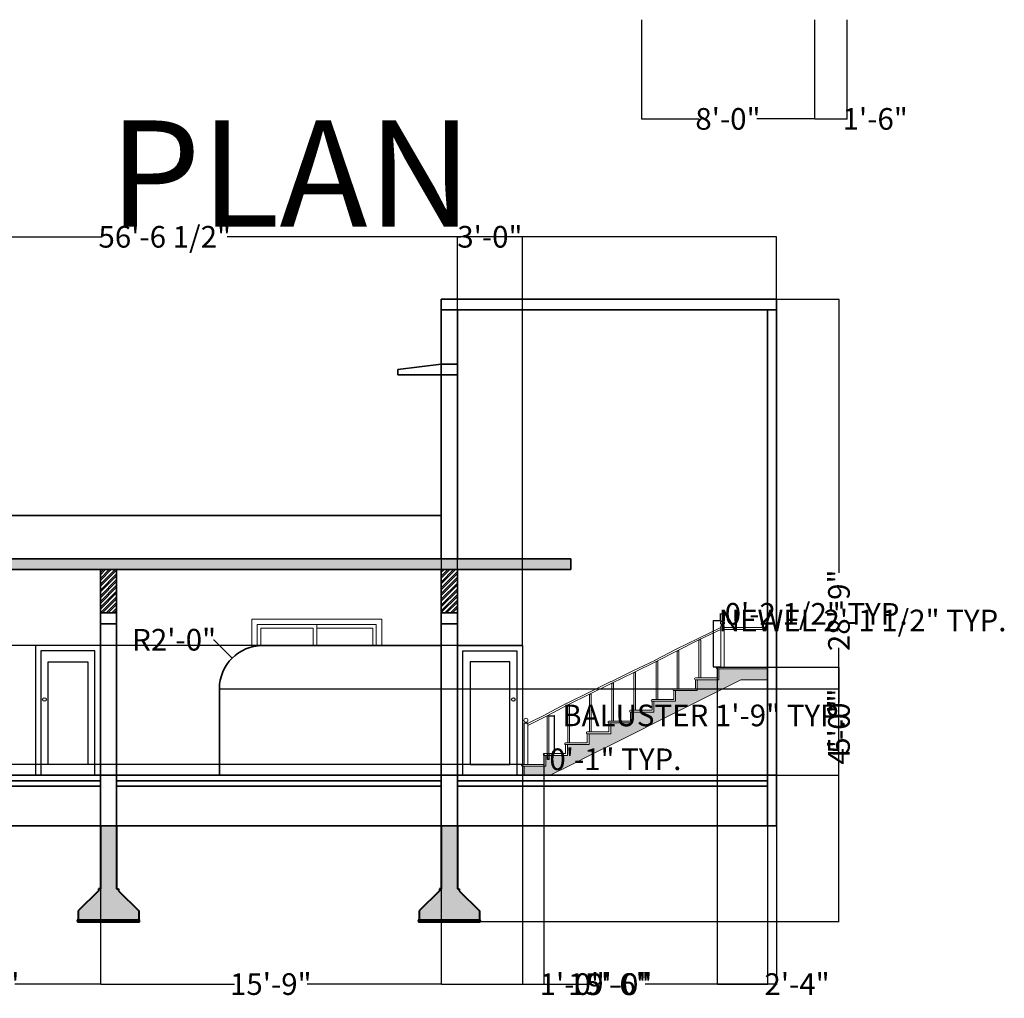
# Model space of a CAD drawing. Units: inches. Extents: x 1146 to 2917, y 889 to 2437.
# Tile 2 of 13: x 1551 to 2097, y 889 to 1432. Entities that reach past the tile are written whole.
import ezdxf

# ---------------------------------------------------------------- set-up
doc = ezdxf.new("R2010")
doc.units = ezdxf.units.IN
doc.header["$MEASUREMENT"] = 0
for name, color, linetype, lineweight in [('A-ANNO-DIMS', 2, 'Continuous', 18), ('A-ANNO-TEXT', 7, 'Continuous', 25), ('A-SECT', 7, 'Continuous', 35), ('A-SECT-PATT', 8, 'Continuous', 13), ('A-SECT-STRS', 6, 'Continuous', 20), ('door', 10, 'Continuous', 25), ('S-FNDN', 7, 'Continuous', 40), ('window', 5, 'Continuous', 18)]:
    doc.layers.add(name, color=color, linetype=linetype, lineweight=lineweight)
doc.styles.get("Standard").update_dxf_attribs({"font": 'arial.ttf'})
doc.dimstyles.get("Standard").update_dxf_attribs({"dimtxt": 12, "dimasz": 0.18, "dimexe": 0.18, "dimexo": 0.0625, "dimgap": 0.09, "dimtad": 0, "dimtoh": 1, "dimdec": 1, "dimzin": 0, "dimdsep": 46, "dimlunit": 4, "dimtxsty": 'Standard', "dimcen": 0.09, "dimadec": 0, "dimazin": 0, "dimtfac": 1, "dimtdec": 1, "dimtofl": 0, "dimtmove": 0, "dimatfit": 3, "dimfxl": 1, "dimtolj": 1, "dimtzin": 0, "dimarcsym": 0})

# ---------------------------------------------------------------- blocks, each defined once
blk = doc.blocks.new('*U61')
blk.add_lwpolyline([(3.12, 0.01), (0.12, 0.01), (0.12, 72.01), (36.12, 72.01), (36.12, 0.01), (33.12, 0.01)])
for points in [[(33.12, 68.99), (33.12, 0.01), (3.12, 0.01), (3.12, 68.99)], [(29.12, 6.01), (29.12, 62.99), (7.12, 62.99), (7.12, 6.01)]]:
    blk.add_lwpolyline(points, close=True)
blk.add_circle((31.12, 42.01), 1)
blk = doc.blocks.new('*U62')
blk.add_lwpolyline([(-6.87, 0.01), (-3.87, 0.01), (-3.87, 72.01), (-39.87, 72.01), (-39.87, 0.01), (-36.87, 0.01)])
for points in [[(-36.87, 68.99), (-36.87, 0.01), (-6.87, 0.01), (-6.87, 68.99)], [(-32.87, 6.01), (-32.87, 62.99), (-10.87, 62.99), (-10.87, 6.01)]]:
    blk.add_lwpolyline(points, close=True)
blk.add_circle((-34.87, 42.01), 1)
blk = doc.blocks.new('RAILING-BALUSTER')
for p, q in [((0, 0), (0, 21)), ((0, 21), (1, 21)), ((1, 21), (1, 0))]:
    blk.add_line(p, q)
blk = doc.blocks.new('RAILING-NEWEL')
for p, q in [((0.13, 23.99), (0.13, 24)), ((0.13, 12), (0.13, 22.87)), ((0.13, 22.87), (2.13, 22.87)), ((0.63, 22.87), (0.63, 23.5)), ((1.63, 22.87), (1.63, 23.5)), ((2.13, 24), (2.13, 23.99)), ((2.13, 22.87), (2.13, 0)), ((0.13, 0), (0.13, 12))]:
    blk.add_line(p, q)
blk.add_circle((1.13, 24.51), 1.13)
blk = doc.blocks.new('*D93')
at = {"layer": 'A-ANNO-DIMS', "color": 0, "lineweight": -2, "transparency": 16777216}
for p, q in [((1844.94, 1045.97), (1848.21, 1045.97)), ((1848.03, 1045.97), (1848.03, 1046.15)), ((1848.03, 1046.15), (1848.21, 1046.15)), ((1848.03, 1025.15), (1848.03, 1045.79)), ((1844.94, 1024.97), (1848.21, 1024.97))]:
    blk.add_line(p, q, dxfattribs=at)
at = {"layer": 'A-ANNO-DIMS', "color": 0, "transparency": 16777216}
for points in [[(1848, 1045.79), (1848.06, 1045.79), (1848.03, 1045.97)], [(1848, 1025.15), (1848.06, 1025.15), (1848.03, 1024.97)]]:
    blk.add_solid(points, dxfattribs=at)
at = {"layer": 'Defpoints', "color": 0, "transparency": 16777216}
for p in [(1844.88, 1045.97), (1848.03, 1045.97), (1844.88, 1024.97)]:
    blk.add_point(p, dxfattribs=at)
at = {"layer": 'A-ANNO-DIMS', "color": 0, "transparency": 16777216, "insert": (1931.19, 1046.15), "char_height": 12, "attachment_point": 5}
blk.add_mtext('\\A1;BALUSTER 1\'-9" TYP.', dxfattribs=at)
blk = doc.blocks.new('*D94')
at = {"layer": 'A-ANNO-DIMS', "color": 0, "lineweight": -2, "transparency": 16777216}
for p, q in [((1843.88, 1024.9), (1843.88, 1021.64)), ((1844.06, 1021.82), (1844.7, 1021.82)), ((1844.88, 1024.9), (1844.88, 1021.64)), ((1844.88, 1021.82), (1845.06, 1021.82))]:
    blk.add_line(p, q, dxfattribs=at)
at = {"layer": 'A-ANNO-DIMS', "color": 0, "transparency": 16777216}
for points in [[(1844.06, 1021.85), (1844.06, 1021.79), (1843.88, 1021.82)], [(1844.7, 1021.85), (1844.7, 1021.79), (1844.88, 1021.82)]]:
    blk.add_solid(points, dxfattribs=at)
at = {"layer": 'Defpoints', "color": 0, "transparency": 16777216}
for p in [(1843.88, 1024.97), (1844.88, 1024.97), (1844.88, 1021.82)]:
    blk.add_point(p, dxfattribs=at)
at = {"layer": 'A-ANNO-DIMS', "color": 0, "transparency": 16777216, "insert": (1881.72, 1021.82), "char_height": 12, "attachment_point": 5}
blk.add_mtext('\\A1;0\'-1" TYP.', dxfattribs=at)
blk = doc.blocks.new('*D95')
at = {"layer": 'A-ANNO-DIMS', "color": 0, "lineweight": -2, "transparency": 16777216}
for p, q in [((1939.92, 1098.61), (1935.95, 1098.61)), ((1936.13, 1098.61), (1936.13, 1098.79)), ((1936.13, 1098.79), (1936.31, 1098.79)), ((1936.13, 1073.15), (1936.13, 1098.43)), ((1939.92, 1072.97), (1935.95, 1072.97))]:
    blk.add_line(p, q, dxfattribs=at)
at = {"layer": 'A-ANNO-DIMS', "color": 0, "transparency": 16777216}
for points in [[(1936.1, 1098.43), (1936.16, 1098.43), (1936.13, 1098.61)], [(1936.1, 1073.15), (1936.16, 1073.15), (1936.13, 1072.97)]]:
    blk.add_solid(points, dxfattribs=at)
at = {"layer": 'Defpoints', "color": 0, "transparency": 16777216}
for p in [(1936.13, 1098.61), (1939.98, 1098.61), (1939.98, 1072.97)]:
    blk.add_point(p, dxfattribs=at)
at = {"layer": 'A-ANNO-DIMS', "color": 0, "transparency": 16777216, "insert": (2018.8, 1098.79), "char_height": 12, "attachment_point": 5}
blk.add_mtext('\\A1;NEWEL 2\'-1 1/2" TYP.', dxfattribs=at)
blk = doc.blocks.new('*D96')
at = {"layer": 'A-ANNO-DIMS', "color": 0, "lineweight": -2, "transparency": 16777216}
for p, q in [((1939.98, 1098.67), (1939.98, 1102.64)), ((1940.16, 1102.46), (1942.06, 1102.46)), ((1942.24, 1098.67), (1942.24, 1102.64)), ((1942.24, 1102.46), (1942.42, 1102.46))]:
    blk.add_line(p, q, dxfattribs=at)
at = {"layer": 'A-ANNO-DIMS', "color": 0, "transparency": 16777216}
for points in [[(1940.16, 1102.49), (1940.16, 1102.43), (1939.98, 1102.46)], [(1942.06, 1102.49), (1942.06, 1102.43), (1942.24, 1102.46)]]:
    blk.add_solid(points, dxfattribs=at)
at = {"layer": 'Defpoints', "color": 0, "transparency": 16777216}
for p in [(1939.98, 1098.61), (1942.24, 1102.46), (1942.24, 1098.61)]:
    blk.add_point(p, dxfattribs=at)
at = {"layer": 'A-ANNO-DIMS', "color": 0, "transparency": 16777216, "insert": (1993.06, 1102.46), "char_height": 12, "attachment_point": 5}
blk.add_mtext('\\A1;0\'-2 1/2" TYP.', dxfattribs=at)
blk = doc.blocks.new('*D141')
at = {"layer": 'A-ANNO-DIMS', "color": 0, "lineweight": -2, "transparency": 16777216}
for p, q in [((1292.5, 931.94), (1292.5, 1311.7)), ((1292.68, 1311.52), (1597.13, 1311.52)), ((1970.95, 1311.52), (1666.5, 1311.52)), ((1971.13, 1277.03), (1971.13, 1311.7))]:
    blk.add_line(p, q, dxfattribs=at)
at = {"layer": 'A-ANNO-DIMS', "color": 0, "transparency": 16777216}
for points in [[(1292.68, 1311.55), (1292.68, 1311.49), (1292.5, 1311.52)], [(1970.95, 1311.55), (1970.95, 1311.49), (1971.13, 1311.52)]]:
    blk.add_solid(points, dxfattribs=at)
at = {"layer": 'Defpoints', "color": 0, "transparency": 16777216}
for p in [(1971.13, 1311.52), (1971.13, 1276.97), (1292.5, 931.87)]:
    blk.add_point(p, dxfattribs=at)
at = {"layer": 'A-ANNO-DIMS', "color": 0, "transparency": 16777216, "insert": (1631.82, 1311.52), "char_height": 12, "attachment_point": 5}
blk.add_mtext('\\A1;56\'-6 1/2"', dxfattribs=at)
blk = doc.blocks.new('*D142')
at = {"layer": 'A-ANNO-DIMS', "color": 0, "lineweight": -2, "transparency": 16777216}
for p, q in [((1785.2, 1276.97), (2005.86, 1276.97)), ((2005.68, 1276.79), (2005.68, 1125.22)), ((2005.68, 932.05), (2005.68, 1083.62)), ((1806.83, 931.87), (2005.86, 931.87))]:
    blk.add_line(p, q, dxfattribs=at)
at = {"layer": 'A-ANNO-DIMS', "color": 0, "transparency": 16777216}
for points in [[(2005.65, 1276.79), (2005.71, 1276.79), (2005.68, 1276.97)], [(2005.65, 932.05), (2005.71, 932.05), (2005.68, 931.87)]]:
    blk.add_solid(points, dxfattribs=at)
at = {"layer": 'Defpoints', "color": 0, "transparency": 16777216}
for p in [(1785.13, 1276.97), (1806.77, 931.87), (2005.68, 931.87)]:
    blk.add_point(p, dxfattribs=at)
at = {"layer": 'A-ANNO-DIMS', "color": 0, "transparency": 16777216, "insert": (2005.68, 1104.42), "char_height": 12, "attachment_point": 5, "rotation": 90}
blk.add_mtext('\\A1;28\'-9"', dxfattribs=at)
blk = doc.blocks.new('*D147')
at = {"layer": 'A-ANNO-DIMS', "color": 0, "lineweight": -2, "transparency": 16777216}
for p, q in [((1461.13, 984.9), (1461.13, 897)), ((1596.13, 984.9), (1596.13, 897)), ((1461.31, 897.18), (1508.5, 897.18)), ((1595.95, 897.18), (1548.77, 897.18))]:
    blk.add_line(p, q, dxfattribs=at)
at = {"layer": 'A-ANNO-DIMS', "color": 0, "transparency": 16777216}
for points in [[(1461.31, 897.21), (1461.31, 897.15), (1461.13, 897.18)], [(1595.95, 897.21), (1595.95, 897.15), (1596.13, 897.18)]]:
    blk.add_solid(points, dxfattribs=at)
at = {"layer": 'Defpoints', "color": 0, "transparency": 16777216}
for p in [(1461.13, 984.97), (1596.13, 984.97), (1596.13, 897.18)]:
    blk.add_point(p, dxfattribs=at)
at = {"layer": 'A-ANNO-DIMS', "color": 0, "transparency": 16777216, "insert": (1528.63, 897.18), "char_height": 12, "attachment_point": 5}
blk.add_mtext('\\A1;11\'-3"', dxfattribs=at)
blk = doc.blocks.new('*D148')
at = {"layer": 'A-ANNO-DIMS', "color": 0, "lineweight": -2, "transparency": 16777216}
for p, q in [((1596.13, 984.9), (1596.13, 897)), ((1785.13, 984.9), (1785.13, 897)), ((1596.31, 897.18), (1670.5, 897.18)), ((1784.95, 897.18), (1710.77, 897.18))]:
    blk.add_line(p, q, dxfattribs=at)
at = {"layer": 'A-ANNO-DIMS', "color": 0, "transparency": 16777216}
for points in [[(1596.31, 897.21), (1596.31, 897.15), (1596.13, 897.18)], [(1784.95, 897.21), (1784.95, 897.15), (1785.13, 897.18)]]:
    blk.add_solid(points, dxfattribs=at)
at = {"layer": 'Defpoints', "color": 0, "transparency": 16777216}
for p in [(1596.13, 984.97), (1785.13, 984.97), (1785.13, 897.18)]:
    blk.add_point(p, dxfattribs=at)
at = {"layer": 'A-ANNO-DIMS', "color": 0, "transparency": 16777216, "insert": (1690.63, 897.18), "char_height": 12, "attachment_point": 5}
blk.add_mtext('\\A1;15\'-9"', dxfattribs=at)
blk = doc.blocks.new('*D149')
at = {"layer": 'A-ANNO-DIMS', "color": 0, "lineweight": -2, "transparency": 16777216}
for p, q in [((1785.13, 1276.9), (1785.13, 897)), ((1971.13, 1276.9), (1971.13, 897)), ((1785.31, 897.18), (1858, 897.18)), ((1970.95, 897.18), (1898.27, 897.18))]:
    blk.add_line(p, q, dxfattribs=at)
at = {"layer": 'A-ANNO-DIMS', "color": 0, "transparency": 16777216}
for points in [[(1785.31, 897.21), (1785.31, 897.15), (1785.13, 897.18)], [(1970.95, 897.21), (1970.95, 897.15), (1971.13, 897.18)]]:
    blk.add_solid(points, dxfattribs=at)
at = {"layer": 'Defpoints', "color": 0, "transparency": 16777216}
for p in [(1785.13, 1276.97), (1971.13, 1276.97), (1971.13, 897.18)]:
    blk.add_point(p, dxfattribs=at)
at = {"layer": 'A-ANNO-DIMS', "color": 0, "transparency": 16777216, "insert": (1878.13, 897.18), "char_height": 12, "attachment_point": 5}
blk.add_mtext('\\A1;15\'-6"', dxfattribs=at)
blk = doc.blocks.new('*D151')
at = {"layer": 'A-ANNO-DIMS', "color": 0, "lineweight": -2, "transparency": 16777216}
for p, q in [((1938.2, 1072.97), (2005.86, 1072.97)), ((2005.68, 1072.79), (2005.68, 1059.01)), ((2005.68, 1013.15), (2005.68, 1026.93)), ((1830.2, 1012.97), (2005.86, 1012.97))]:
    blk.add_line(p, q, dxfattribs=at)
at = {"layer": 'A-ANNO-DIMS', "color": 0, "transparency": 16777216}
for points in [[(2005.65, 1072.79), (2005.71, 1072.79), (2005.68, 1072.97)], [(2005.65, 1013.15), (2005.71, 1013.15), (2005.68, 1012.97)]]:
    blk.add_solid(points, dxfattribs=at)
at = {"layer": 'Defpoints', "color": 0, "transparency": 16777216}
for p in [(1938.13, 1072.97), (2005.68, 1072.97), (1830.13, 1012.97)]:
    blk.add_point(p, dxfattribs=at)
at = {"layer": 'A-ANNO-DIMS', "color": 0, "transparency": 16777216, "insert": (2005.68, 1042.97), "char_height": 12, "attachment_point": 5, "rotation": 90}
blk.add_mtext('\\A1;5\'-0"', dxfattribs=at)
blk = doc.blocks.new('*D152')
at = {"layer": 'A-ANNO-DIMS', "color": 0, "lineweight": -2, "transparency": 16777216}
for p, q in [((1938.13, 1072.9), (1938.13, 897)), ((1830.13, 1012.9), (1830.13, 897)), ((1830.31, 897.18), (1868.09, 897.18)), ((1937.95, 897.18), (1900.17, 897.18))]:
    blk.add_line(p, q, dxfattribs=at)
at = {"layer": 'A-ANNO-DIMS', "color": 0, "transparency": 16777216}
for points in [[(1830.31, 897.21), (1830.31, 897.15), (1830.13, 897.18)], [(1937.95, 897.21), (1937.95, 897.15), (1938.13, 897.18)]]:
    blk.add_solid(points, dxfattribs=at)
at = {"layer": 'Defpoints', "color": 0, "transparency": 16777216}
for p in [(1938.13, 1072.97), (1830.13, 1012.97), (1938.13, 897.18)]:
    blk.add_point(p, dxfattribs=at)
at = {"layer": 'A-ANNO-DIMS', "color": 0, "transparency": 16777216, "insert": (1884.13, 897.18), "char_height": 12, "attachment_point": 5}
blk.add_mtext('\\A1;9\'-0"', dxfattribs=at)
blk = doc.blocks.new('*D153')
at = {"layer": 'A-ANNO-DIMS', "color": 0, "lineweight": -2, "transparency": 16777216}
for p, q in [((1938.13, 1072.9), (1938.13, 897)), ((1966.13, 1072.9), (1966.13, 897)), ((1938.31, 897.18), (1965.95, 897.18)), ((1966.13, 897.18), (1966.31, 897.18))]:
    blk.add_line(p, q, dxfattribs=at)
at = {"layer": 'A-ANNO-DIMS', "color": 0, "transparency": 16777216}
for points in [[(1938.31, 897.21), (1938.31, 897.15), (1938.13, 897.18)], [(1965.95, 897.21), (1965.95, 897.15), (1966.13, 897.18)]]:
    blk.add_solid(points, dxfattribs=at)
at = {"layer": 'Defpoints', "color": 0, "transparency": 16777216}
for p in [(1938.13, 1072.97), (1966.13, 1072.97), (1966.13, 897.18)]:
    blk.add_point(p, dxfattribs=at)
at = {"layer": 'A-ANNO-DIMS', "color": 0, "transparency": 16777216, "insert": (1982.46, 897.18), "char_height": 12, "attachment_point": 5}
blk.add_mtext('\\A1;2\'-4"', dxfattribs=at)
blk = doc.blocks.new('*D154')
at = {"layer": 'A-ANNO-DIMS', "color": 0, "lineweight": -2, "transparency": 16777216}
for p, q in [((1830.07, 1018.97), (1257.62, 1018.97)), ((1257.8, 1018.97), (1257.8, 1019.15)), ((1257.8, 1019.15), (1257.98, 1019.15)), ((1257.8, 1013.15), (1257.8, 1018.79)), ((1830.07, 1012.97), (1257.62, 1012.97))]:
    blk.add_line(p, q, dxfattribs=at)
at = {"layer": 'A-ANNO-DIMS', "color": 0, "transparency": 16777216}
for points in [[(1257.77, 1018.79), (1257.83, 1018.79), (1257.8, 1018.97)], [(1257.77, 1013.15), (1257.83, 1013.15), (1257.8, 1012.97)]]:
    blk.add_solid(points, dxfattribs=at)
at = {"layer": 'Defpoints', "color": 0, "transparency": 16777216}
for p in [(1257.8, 1018.97), (1830.13, 1018.97), (1830.13, 1012.97)]:
    blk.add_point(p, dxfattribs=at)
at = {"layer": 'A-ANNO-DIMS', "color": 0, "transparency": 16777216, "insert": (1274.02, 1019.15), "char_height": 12, "attachment_point": 5}
blk.add_mtext('\\A1;0\'-6"', dxfattribs=at)
blk = doc.blocks.new('*D155')
at = {"layer": 'A-ANNO-DIMS', "color": 0, "lineweight": -2, "transparency": 16777216}
for p, q in [((1842.13, 1024.9), (1842.13, 897)), ((1830.13, 1018.9), (1830.13, 897)), ((1830.31, 897.18), (1841.95, 897.18)), ((1842.13, 897.18), (1842.31, 897.18))]:
    blk.add_line(p, q, dxfattribs=at)
at = {"layer": 'A-ANNO-DIMS', "color": 0, "transparency": 16777216}
for points in [[(1830.31, 897.21), (1830.31, 897.15), (1830.13, 897.18)], [(1841.95, 897.21), (1841.95, 897.15), (1842.13, 897.18)]]:
    blk.add_solid(points, dxfattribs=at)
at = {"layer": 'Defpoints', "color": 0, "transparency": 16777216}
for p in [(1842.13, 1024.97), (1830.13, 1018.97), (1842.13, 897.18)]:
    blk.add_point(p, dxfattribs=at)
at = {"layer": 'A-ANNO-DIMS', "color": 0, "transparency": 16777216, "insert": (1857.79, 897.18), "char_height": 12, "attachment_point": 5}
blk.add_mtext('\\A1;1\'-0"', dxfattribs=at)
blk = doc.blocks.new('*D156')
at = {"layer": 'A-ANNO-DIMS', "color": 0, "lineweight": -2, "transparency": 16777216}
for p, q in [((1794.13, 1085.03), (1794.13, 1311.7)), ((1794.31, 1311.52), (1796.1, 1311.52)), ((1829.95, 1311.52), (1828.17, 1311.52)), ((1830.13, 1085.03), (1830.13, 1311.7))]:
    blk.add_line(p, q, dxfattribs=at)
at = {"layer": 'A-ANNO-DIMS', "color": 0, "transparency": 16777216}
for points in [[(1794.31, 1311.55), (1794.31, 1311.49), (1794.13, 1311.52)], [(1829.95, 1311.55), (1829.95, 1311.49), (1830.13, 1311.52)]]:
    blk.add_solid(points, dxfattribs=at)
at = {"layer": 'Defpoints', "color": 0, "transparency": 16777216}
for p in [(1830.13, 1311.52), (1794.13, 1084.97), (1830.13, 1084.97)]:
    blk.add_point(p, dxfattribs=at)
at = {"layer": 'A-ANNO-DIMS', "color": 0, "transparency": 16777216, "insert": (1812.13, 1311.52), "char_height": 12, "attachment_point": 5}
blk.add_mtext('\\A1;3\'-0"', dxfattribs=at)
blk = doc.blocks.new('*D157')
at = {"layer": 'A-ANNO-DIMS', "color": 0, "lineweight": -2, "transparency": 16777216}
for p, q in [((1830.07, 1084.97), (1257.62, 1084.97)), ((1257.8, 1084.79), (1257.8, 1065.04)), ((1257.8, 1013.15), (1257.8, 1032.89)), ((1830.07, 1012.97), (1257.62, 1012.97))]:
    blk.add_line(p, q, dxfattribs=at)
at = {"layer": 'A-ANNO-DIMS', "color": 0, "transparency": 16777216}
for points in [[(1257.77, 1084.79), (1257.83, 1084.79), (1257.8, 1084.97)], [(1257.77, 1013.15), (1257.83, 1013.15), (1257.8, 1012.97)]]:
    blk.add_solid(points, dxfattribs=at)
at = {"layer": 'Defpoints', "color": 0, "transparency": 16777216}
for p in [(1257.8, 1084.97), (1830.13, 1084.97), (1830.13, 1012.97)]:
    blk.add_point(p, dxfattribs=at)
at = {"layer": 'A-ANNO-DIMS', "color": 0, "transparency": 16777216, "insert": (1257.8, 1048.97), "char_height": 12, "attachment_point": 5, "rotation": 90}
blk.add_mtext('\\A1;6\'-0"', dxfattribs=at)
blk = doc.blocks.new('*D161')
at = {"layer": 'A-ANNO-DIMS', "color": 0, "lineweight": -2, "transparency": 16777216}
for p, q in [((1662.2, 1060.94), (2005.86, 1060.94)), ((2005.68, 1060.76), (2005.68, 1053.24)), ((2005.68, 1013.15), (2005.68, 1020.67)), ((1662.2, 1012.97), (2005.86, 1012.97))]:
    blk.add_line(p, q, dxfattribs=at)
at = {"layer": 'A-ANNO-DIMS', "color": 0, "transparency": 16777216}
for points in [[(2005.65, 1060.76), (2005.71, 1060.76), (2005.68, 1060.94)], [(2005.65, 1013.15), (2005.71, 1013.15), (2005.68, 1012.97)]]:
    blk.add_solid(points, dxfattribs=at)
at = {"layer": 'Defpoints', "color": 0, "transparency": 16777216}
for p in [(1662.13, 1060.94), (2005.68, 1060.94), (1662.13, 1012.97)]:
    blk.add_point(p, dxfattribs=at)
at = {"layer": 'A-ANNO-DIMS', "color": 0, "transparency": 16777216, "insert": (2005.68, 1036.96), "char_height": 12, "attachment_point": 5, "rotation": 90}
blk.add_mtext('\\A1;4\'-0"', dxfattribs=at)
blk = doc.blocks.new('*D166')
at = {"layer": 'A-ANNO-DIMS', "color": 0, "lineweight": -2, "transparency": 16777216}
for p, q in [((1896.13, 1431.83), (1896.13, 1376.71)), ((1992.13, 1431.83), (1992.13, 1376.71)), ((1896.31, 1376.89), (1928.09, 1376.89)), ((1991.95, 1376.89), (1960.18, 1376.89))]:
    blk.add_line(p, q, dxfattribs=at)
at = {"layer": 'A-ANNO-DIMS', "color": 0, "transparency": 16777216}
for points in [[(1896.31, 1376.92), (1896.31, 1376.86), (1896.13, 1376.89)], [(1991.95, 1376.92), (1991.95, 1376.86), (1992.13, 1376.89)]]:
    blk.add_solid(points, dxfattribs=at)
at = {"layer": 'Defpoints', "color": 0, "transparency": 16777216}
for p in [(1896.13, 1431.89), (1992.13, 1431.89), (1992.13, 1376.89)]:
    blk.add_point(p, dxfattribs=at)
at = {"layer": 'A-ANNO-DIMS', "color": 0, "transparency": 16777216, "insert": (1944.13, 1376.89), "char_height": 12, "attachment_point": 5}
blk.add_mtext('\\A1;8\'-0"', dxfattribs=at)
blk = doc.blocks.new('*D167')
at = {"layer": 'A-ANNO-DIMS', "color": 0, "lineweight": -2, "transparency": 16777216}
for p, q in [((1992.13, 1431.83), (1992.13, 1376.71)), ((2010.13, 1431.83), (2010.13, 1376.71)), ((1992.31, 1376.89), (2009.95, 1376.89)), ((2010.13, 1376.89), (2010.31, 1376.89))]:
    blk.add_line(p, q, dxfattribs=at)
at = {"layer": 'A-ANNO-DIMS', "color": 0, "transparency": 16777216}
for points in [[(1992.31, 1376.92), (1992.31, 1376.86), (1992.13, 1376.89)], [(2009.95, 1376.92), (2009.95, 1376.86), (2010.13, 1376.89)]]:
    blk.add_solid(points, dxfattribs=at)
at = {"layer": 'Defpoints', "color": 0, "transparency": 16777216}
for p in [(1992.13, 1431.89), (2010.13, 1431.89), (2010.13, 1376.89)]:
    blk.add_point(p, dxfattribs=at)
at = {"layer": 'A-ANNO-DIMS', "color": 0, "transparency": 16777216, "insert": (2025.79, 1376.89), "char_height": 12, "attachment_point": 5}
blk.add_mtext('\\A1;1\'-6"', dxfattribs=at)
blk = doc.blocks.new('*D174')
at = {"layer": 'A-ANNO-DIMS', "color": 0, "lineweight": -2, "transparency": 16777216}
for p, q in [((1658.8, 1088.1), (1658.98, 1088.1)), ((1658.98, 1088.1), (1669.04, 1078.04)), ((1686.04, 1060.94), (1686.22, 1060.94)), ((1686.13, 1060.85), (1686.13, 1061.03))]:
    blk.add_line(p, q, dxfattribs=at)
at = {"layer": 'A-ANNO-DIMS', "color": 0, "transparency": 16777216}
blk.add_solid([(1669.06, 1078.06), (1669.01, 1078.02), (1669.16, 1077.91)], dxfattribs=at)
at = {"layer": 'Defpoints', "color": 0, "transparency": 16777216}
for p in [(1669.16, 1077.91), (1686.13, 1060.94)]:
    blk.add_point(p, dxfattribs=at)
at = {"layer": 'A-ANNO-DIMS', "color": 0, "transparency": 16777216, "insert": (1637.02, 1088.1), "char_height": 12, "attachment_point": 5}
blk.add_mtext('\\A1;R2\'-0"', dxfattribs=at)

msp = doc.modelspace()

# ---------------------------------------------------------------- hatches: boundary and pattern name
at = {"layer": 'A-SECT-PATT'}
h = msp.add_hatch(dxfattribs=at)
h.set_pattern_fill('ANSI32', color=256, scale=6)
h.paths.add_polyline_path([(1605.13, 1126.97), (1596.13, 1126.97), (1596.13, 1102.97), (1605.13, 1102.97)])
h.paths.add_polyline_path([(1794.13, 1126.97), (1785.13, 1126.97), (1785.13, 1102.97), (1794.13, 1102.97)])
h.paths.add_polyline_path([(1470.13, 1126.97), (1461.13, 1126.97), (1461.13, 1096.97), (1470.13, 1096.97)])
h.paths.add_polyline_path([(1461.13, 1132.97), (1465.63, 1132.97), (1465.63, 1156.97), (1461.13, 1156.97)])
h = msp.add_hatch(dxfattribs=at)
h.set_pattern_fill('AR-CONC', color=256, scale=0.3)
h.set_pattern_definition([(50, (0, 0), (2.1517805, -0.1882564), [0.225, -2.475]), (355, (0, 0), (-0.416254, 2.2565764), [0.18, -1.98]), (100.45144, (0.1793, -0.0157), (1.7355265, 2.06832), [0.1912206, -2.1034263]), (46.1842, (0, 0.6), (3.201724, -0.496558), [0.3375, -3.7125]), (96.63564, (0.2668, 0.5586), (2.803986, 2.922356), [0.286831, -3.1551413]), (351.18416, (0, 0.6), (2.803986, 2.922356), [0.27, -2.97]), (21, (0.3, 0.45), (1.7907212, -1.2078567), [0.225, -2.475]), (326, (0.3, 0.45), (0.729946, 2.1754501), [0.18, -1.98]), (71.45144, (0.4492, 0.3493), (2.5206671, 0.9675935), [0.1912206, -2.1034263]), (37.5, (0, 0), (0.03647957, 0.99868156), [0, -1.956, 0, -2.01, 0, -1.9875]), (7.5, (0, 0), (0.7892086, 1.18323514), [0, -1.146, 0, -1.911, 0, -0.7575]), (327.5, (-0.669, 0), (1.6014673, -0.06766462), [0, -0.75, 0, -2.34, 0, -3.105]), (317.5, (-0.969, 0), (1.7495585, 0.30031495), [0, -0.975, 0, -1.554, 0, -2.205])])
h.paths.add_polyline_path([(1856.99, 1126.97), (1856.99, 1132.97), (1461.13, 1132.97), (1461.13, 1126.97)])
h = msp.add_hatch(dxfattribs=at)
h.set_pattern_fill('AR-CONC', color=256, scale=0.8)
h.set_pattern_definition([(50, (0, 0), (5.738081, -0.502017), [0.6, -6.6]), (355, (0, 0), (-1.11001, 6.017537), [0.48, -5.28]), (100.45144, (0.478, -0.042), (4.628071, 5.51552), [0.509922, -5.609137]), (46.1842, (0, 1.6), (8.53793, -1.324154), [0.9, -9.9]), (96.63564, (0.7115, 1.49), (7.477296, 7.79295), [0.764883, -8.41371]), (351.18416, (0, 1.6), (7.477296, 7.79295), [0.72, -7.92]), (21, (0.8, 1.2), (4.775256, -3.220951), [0.6, -6.6]), (326, (0.8, 1.2), (1.946523, 5.8012), [0.48, -5.28]), (71.45144, (1.198, 0.9316), (6.721779, 2.580249), [0.509922, -5.609137]), (37.5, (0, 0), (0.0972788, 2.6631508), [0, -5.216, 0, -5.36, 0, -5.3]), (7.5, (0, 0), (2.1045563, 3.1552937), [0, -3.056, 0, -5.096, 0, -2.02]), (327.5, (-1.784, 0), (4.2705795, -0.180439), [0, -2, 0, -6.24, 0, -8.28]), (317.5, (-2.584, 0), (4.6654894, 0.80084), [0, -2.6, 0, -4.144, 0, -5.88])])
h.paths.add_polyline_path([(1916.82, 1048.6), (1951.34, 1065.86, -0.116434), (1951.79, 1065.97), (1966.13, 1065.97), (1966.13, 1071.97), (1939.13, 1071.97), (1939.13, 1065.97), (1927.13, 1065.97), (1927.13, 1059.97), (1915.13, 1059.97), (1915.13, 1053.97), (1903.13, 1053.97), (1903.13, 1047.97), (1891.13, 1047.97), (1891.13, 1041.97), (1879.13, 1041.97), (1879.13, 1035.97), (1867.13, 1035.97), (1867.13, 1029.97), (1855.13, 1029.97), (1855.13, 1023.97), (1843.13, 1023.97), (1843.13, 1017.97), (1831.13, 1017.97), (1831.13, 1012.97), (1845.55, 1012.97), (1856.82, 1018.6), (1868.82, 1024.6), (1880.82, 1030.6)])
h = msp.add_hatch(dxfattribs=at)
h.set_pattern_fill('AR-CONC', color=256, scale=0.3)
h.set_pattern_definition([(50, (291, 0), (2.1517805, -0.1882564), [0.225, -2.475]), (355, (291, 0), (-0.416254, 2.2565764), [0.18, -1.98]), (100.45144, (291.1793, -0.0157), (1.7355265, 2.06832), [0.1912206, -2.1034263]), (46.1842, (291, 0.6), (3.201724, -0.496558), [0.3375, -3.7125]), (96.63564, (291.2668, 0.5586), (2.803986, 2.922356), [0.286831, -3.155141]), (351.18416, (291, 0.6), (2.803986, 2.922356), [0.27, -2.97]), (21, (291.3, 0.45), (1.7907212, -1.2078567), [0.225, -2.475]), (326, (291.3, 0.45), (0.729946, 2.17545), [0.18, -1.98]), (71.45144, (291.4492, 0.3493), (2.520667, 0.9675935), [0.1912206, -2.1034263]), (37.5, (291, 0), (0.03647957, 0.99868156), [0, -1.956, 0, -2.01, 0, -1.9875]), (7.5, (291, 0), (0.7892086, 1.18323514), [0, -1.146, 0, -1.911, 0, -0.7575]), (327.5, (290.331, 0), (1.6014673, -0.0676646), [0, -0.75, 0, -2.34, 0, -3.105]), (317.5, (290.031, 0), (1.7495585, 0.300315), [0, -0.975, 0, -1.554, 0, -2.205])])
h.paths.add_polyline_path([(1606.13, 948.97), (1606.13, 949.97), (1605.13, 949.97), (1605.13, 984.97), (1596.13, 984.97), (1596.13, 949.97), (1595.13, 949.97), (1595.13, 948.97), (1583.85, 937.8), (1583.85, 932.73), (1617.42, 932.73), (1617.42, 937.8)])
h = msp.add_hatch(dxfattribs=at)
h.set_pattern_fill('AR-CONC', color=256, scale=0.3)
h.set_pattern_definition([(50, (480, 0), (2.1517805, -0.1882564), [0.225, -2.475]), (355, (480, 0), (-0.416254, 2.2565764), [0.18, -1.98]), (100.45144, (480.1793, -0.0157), (1.7355265, 2.06832), [0.1912206, -2.1034263]), (46.1842, (480, 0.6), (3.201724, -0.496558), [0.3375, -3.7125]), (96.63564, (480.2668, 0.5586), (2.803986, 2.922356), [0.286831, -3.155141]), (351.18416, (480, 0.6), (2.803986, 2.922356), [0.27, -2.97]), (21, (480.3, 0.45), (1.7907212, -1.2078567), [0.225, -2.475]), (326, (480.3, 0.45), (0.729946, 2.17545), [0.18, -1.98]), (71.45144, (480.4492, 0.3493), (2.520667, 0.9675935), [0.1912206, -2.1034263]), (37.5, (480, 0), (0.03647957, 0.99868156), [0, -1.956, 0, -2.01, 0, -1.9875]), (7.5, (480, 0), (0.7892086, 1.18323514), [0, -1.146, 0, -1.911, 0, -0.7575]), (327.5, (479.331, 0), (1.6014673, -0.0676646), [0, -0.75, 0, -2.34, 0, -3.105]), (317.5, (479.031, 0), (1.7495585, 0.300315), [0, -0.975, 0, -1.554, 0, -2.205])])
h.paths.add_polyline_path([(1795.13, 948.97), (1795.13, 949.97), (1794.13, 949.97), (1794.13, 984.97), (1785.13, 984.97), (1785.13, 949.97), (1784.13, 949.97), (1784.13, 948.97), (1772.85, 937.8), (1772.85, 932.73), (1806.42, 932.73), (1806.42, 937.8)])

# ---------------------------------------------------------------- linework, layer by layer
at = {"layer": 'A-SECT'}
for p, q in [((1785.13, 1276.97), (1971.13, 1276.97)), ((1785.13, 1132.97), (1785.13, 1276.97)), ((1971.13, 984.97), (1971.13, 1276.97)), ((1785.13, 1270.97), (1971.13, 1270.97)), ((1794.13, 1132.97), (1794.13, 1270.97)), ((1966.13, 984.97), (1966.13, 1270.97)), ((1761.13, 1237.97), (1785.13, 1240.97)), ((1785.13, 1240.97), (1794.13, 1240.97)), ((1761.13, 1234.97), (1761.13, 1237.97)), ((1785.13, 1234.97), (1761.13, 1234.97)), ((1785.13, 1234.97), (1794.13, 1234.97)), ((1461.13, 1156.97), (1785.13, 1156.97)), ((1461.13, 1132.97), (1856.99, 1132.97)), ((1856.99, 1132.97), (1856.99, 1126.97)), ((1461.13, 1126.97), (1856.99, 1126.97)), ((1596.13, 984.97), (1596.13, 1126.97)), ((1605.13, 984.97), (1605.13, 1126.97)), ((1785.13, 984.97), (1785.13, 1126.97)), ((1794.13, 984.97), (1794.13, 1126.97)), ((1596.13, 1102.97), (1605.13, 1102.97)), ((1785.13, 1102.97), (1794.13, 1102.97)), ((1596.13, 1096.97), (1605.13, 1096.97)), ((1785.13, 1096.97), (1794.13, 1096.97)), ((1785.13, 1084.94), (1686.13, 1084.94)), ((1662.13, 1060.94), (1662.13, 1012.97)), ((1638.13, 1012.97), (1431.13, 1012.97)), ((1470.13, 1012.97), (1971.13, 1012.97)), ((1470.13, 1009.97), (1596.13, 1009.97)), ((1470.13, 1006.97), (1596.13, 1006.97)), ((1605.13, 1009.97), (1785.13, 1009.97)), ((1605.13, 1009.97), (1638.13, 1009.97)), ((1605.13, 1006.97), (1785.13, 1006.97)), ((1605.13, 1006.97), (1638.13, 1006.97)), ((1794.13, 1009.97), (1966.13, 1009.97)), ((1794.13, 1006.97), (1966.13, 1006.97)), ((1461.13, 984.97), (1971.13, 984.97))]:
    msp.add_line(p, q, dxfattribs=at)
msp.add_arc((1686.13, 1060.94), 24, 90, 180, dxfattribs=at)
at = {"layer": 'A-SECT-STRS'}
for p, q in [((1927.57, 1088.87), (1940.11, 1094.91)), ((1928.01, 1087.97), (1940.11, 1093.8)), ((1942.11, 1094.82), (1966.13, 1094.82)), ((1942.11, 1093.82), (1966.13, 1093.82)), ((1915.44, 1082.86), (1927.56, 1088.86)), ((1915.89, 1081.97), (1928.01, 1087.97)), ((1903.87, 1076.85), (1915.43, 1082.85)), ((1904.34, 1075.97), (1915.89, 1081.97)), ((1891.47, 1070.87), (1903.9, 1076.87)), ((1891.91, 1069.97), (1904.34, 1075.97)), ((1879.26, 1064.86), (1891.47, 1070.86)), ((1938.13, 1072.97), (1966.13, 1072.97)), ((1938.13, 1066.97), (1938.13, 1071.97)), ((1938.13, 1071.97), (1966.13, 1071.97)), ((1939.13, 1065.97), (1939.13, 1071.97)), ((1866.92, 1058.87), (1879.26, 1064.87)), ((1879.7, 1063.97), (1891.91, 1069.97)), ((1916.82, 1048.6), (1951.34, 1065.86)), ((1926.13, 1066.97), (1938.13, 1066.97)), ((1926.13, 1060.97), (1926.13, 1065.97)), ((1926.13, 1065.97), (1939.13, 1065.97)), ((1927.13, 1059.97), (1927.13, 1065.97)), ((1951.79, 1065.97), (1966.13, 1065.97)), ((1867.36, 1057.97), (1879.7, 1063.97)), ((1914.13, 1060.97), (1926.13, 1060.97)), ((1914.13, 1054.97), (1914.13, 1059.97)), ((1914.13, 1059.97), (1927.13, 1059.97)), ((1915.13, 1053.97), (1915.13, 1059.97)), ((1854.89, 1052.86), (1866.91, 1058.86)), ((1855.34, 1051.97), (1867.36, 1057.97)), ((1902.13, 1054.97), (1914.13, 1054.97)), ((1902.13, 1048.97), (1902.13, 1053.97)), ((1902.13, 1053.97), (1915.13, 1053.97)), ((1903.13, 1047.97), (1903.13, 1053.97)), ((1843.42, 1046.85), (1854.87, 1052.85)), ((1843.88, 1045.97), (1855.34, 1051.97)), ((1880.82, 1030.6), (1916.82, 1048.6)), ((1890.13, 1048.97), (1902.13, 1048.97)), ((1832.66, 1041.53), (1843.44, 1046.86)), ((1833.1, 1040.64), (1843.88, 1045.97)), ((1878.13, 1042.97), (1890.13, 1042.97)), ((1890.13, 1042.97), (1890.13, 1047.97)), ((1890.13, 1047.97), (1903.13, 1047.97)), ((1891.13, 1041.97), (1891.13, 1047.97)), ((1878.13, 1036.97), (1878.13, 1041.97)), ((1878.13, 1041.97), (1891.13, 1041.97)), ((1879.13, 1035.97), (1879.13, 1041.97)), ((1866.13, 1036.97), (1878.13, 1036.97)), ((1866.13, 1030.97), (1866.13, 1035.97)), ((1866.13, 1035.97), (1879.13, 1035.97)), ((1867.13, 1029.97), (1867.13, 1035.97)), ((1854.13, 1030.97), (1866.13, 1030.97)), ((1854.13, 1024.97), (1854.13, 1029.97)), ((1854.13, 1029.97), (1867.13, 1029.97)), ((1855.13, 1023.97), (1855.13, 1029.97)), ((1868.82, 1024.6), (1880.82, 1030.6)), ((1842.13, 1024.97), (1854.13, 1024.97)), ((1842.13, 1018.97), (1842.13, 1023.97)), ((1842.13, 1023.97), (1855.13, 1023.97)), ((1843.13, 1017.97), (1843.13, 1023.97)), ((1856.82, 1018.6), (1868.82, 1024.6)), ((1830.13, 1018.97), (1842.13, 1018.97)), ((1830.13, 1012.97), (1830.13, 1017.97)), ((1830.13, 1017.97), (1843.13, 1017.97)), ((1831.13, 1012.97), (1831.13, 1017.97)), ((1845.55, 1012.97), (1856.82, 1018.6))]:
    msp.add_line(p, q, dxfattribs=at)
for centre, radius, end in [((1938.13, 1072.47), 0.5, 270), ((1926.13, 1066.47), 0.5, 270), ((1951.79, 1064.97), 1, 116.5651), ((1914.13, 1060.47), 0.5, 270), ((1902.13, 1054.47), 0.5, 270), ((1890.13, 1048.47), 0.5, 270), ((1878.13, 1042.47), 0.5, 270), ((1866.13, 1036.47), 0.5, 270), ((1854.13, 1030.47), 0.5, 270), ((1842.13, 1024.47), 0.5, 270), ((1830.13, 1018.47), 0.5, 270)]:
    msp.add_arc(centre, radius, 90, end, dxfattribs=at)
at = {"layer": 'S-FNDN'}
for p, q in [((1596.13, 984.97), (1596.13, 949.97)), ((1605.13, 984.97), (1605.13, 949.97)), ((1785.13, 984.97), (1785.13, 949.97)), ((1794.13, 984.97), (1794.13, 949.97)), ((1595.13, 948.97), (1583.85, 937.8)), ((1596.13, 949.97), (1595.13, 949.97)), ((1595.13, 949.97), (1595.13, 948.97)), ((1605.13, 949.97), (1606.13, 949.97)), ((1606.13, 949.97), (1606.13, 948.97)), ((1606.13, 948.97), (1617.42, 937.8)), ((1784.13, 948.97), (1772.85, 937.8)), ((1785.13, 949.97), (1784.13, 949.97)), ((1784.13, 949.97), (1784.13, 948.97)), ((1794.13, 949.97), (1795.13, 949.97)), ((1795.13, 949.97), (1795.13, 948.97)), ((1795.13, 948.97), (1806.42, 937.8)), ((1583.85, 937.8), (1583.85, 932.73)), ((1617.42, 937.8), (1617.42, 932.73)), ((1772.85, 937.8), (1772.85, 932.73)), ((1806.42, 937.8), (1806.42, 932.73)), ((1583.85, 932.73), (1617.42, 932.73)), ((1583.85, 931.73), (1617.42, 931.73)), ((1772.85, 932.73), (1806.42, 932.73)), ((1772.85, 931.73), (1806.42, 931.73))]:
    msp.add_line(p, q, dxfattribs=at)
for centre, start, end in [((1583.85, 932.23), 90, 270), ((1617.42, 932.23), 270, 90), ((1772.85, 932.23), 90, 270), ((1806.42, 932.23), 270, 90)]:
    msp.add_arc(centre, 0.5, start, end, dxfattribs=at)
at = {"layer": 'window'}
for p, q in [((1683.13, 1084.76), (1683.13, 1096.48)), ((1683.13, 1096.48), (1716.13, 1096.48)), ((1716.13, 1096.48), (1749.13, 1096.48)), ((1716.13, 1084.94), (1716.13, 1096.48)), ((1749.13, 1096.48), (1749.13, 1084.94))]:
    msp.add_line(p, q, dxfattribs=at)
for points in [[(1680.13, 1084.18), (1680.13, 1099.48), (1752.13, 1099.48), (1752.13, 1084.94)], [(1685.13, 1084.92), (1685.13, 1094.48), (1714.13, 1094.48)], [(1714.13, 1094.48), (1714.13, 1084.94)], [(1716.13, 1094.48), (1747.13, 1094.48), (1747.13, 1084.94)]]:
    msp.add_lwpolyline(points, dxfattribs=at)

# ---------------------------------------------------------------- block references
at = {"layer": 'A-SECT-STRS'}
for name, p in [('RAILING-NEWEL', (1939.98, 1072.97)), ('RAILING-BALUSTER', (1928.01, 1066.97)), ('RAILING-BALUSTER', (1915.89, 1060.97)), ('RAILING-BALUSTER', (1904.34, 1054.97)), ('RAILING-BALUSTER', (1891.91, 1048.97)), ('RAILING-BALUSTER', (1879.7, 1042.97)), ('RAILING-BALUSTER', (1867.36, 1036.97)), ('RAILING-BALUSTER', (1855.34, 1030.97)), ('RAILING-NEWEL', (1830.97, 1018.97)), ('RAILING-BALUSTER', (1843.88, 1024.97))]:
    msp.add_blockref(name, p, dxfattribs=at)
at = {"layer": 'door'}
for name, p in [('*U62', (1600, 1012.95)), ('*U61', (1794.01, 1012.95))]:
    msp.add_blockref(name, p, dxfattribs=at)

# ---------------------------------------------------------------- texts
at = {"layer": 'A-ANNO-TEXT', "insert": (1600.88, 1376.03), "char_height": 58.92, "attachment_point": 1}
msp.add_mtext_dynamic_manual_height_columns('PLAN', width=2144.5264, gutter_width=2.95, heights=[0], dxfattribs=at)

# ---------------------------------------------------------------- dimensions: what is measured, and where the dimension line sits
at = {"layer": 'A-ANNO-DIMS'}
for base, p1, p2, picture, middle in [((1992.13, 1376.89), (1896.13, 1431.89), (1992.13, 1431.89), '*D166', (1944.13, 1376.89)), ((2010.13, 1376.89), (1992.13, 1431.89), (2010.13, 1431.89), '*D167', (2025.79, 1376.89)), ((1971.13, 1311.52), (1292.5, 931.87), (1971.13, 1276.97), '*D141', (1631.82, 1311.52)), ((1830.13, 1311.52), (1794.13, 1084.97), (1830.13, 1084.97), '*D156', (1812.13, 1311.52)), ((1971.13, 897.18), (1785.13, 1276.97), (1971.13, 1276.97), '*D149', (1878.13, 897.18)), ((1938.13, 897.18), (1830.13, 1012.97), (1938.13, 1072.97), '*D152', (1884.13, 897.18)), ((1966.13, 897.18), (1938.13, 1072.97), (1966.13, 1072.97), '*D153', (1982.46, 897.18)), ((1842.13, 897.18), (1830.13, 1018.97), (1842.13, 1024.97), '*D155', (1857.79, 897.18)), ((1596.13, 897.18), (1461.13, 984.97), (1596.13, 984.97), '*D147', (1528.63, 897.18)), ((1785.13, 897.18), (1596.13, 984.97), (1785.13, 984.97), '*D148', (1690.63, 897.18))]:
    dim = msp.add_linear_dim(base=base, p1=p1, p2=p2, dimstyle='Standard', override={"dimdec": 1, "dimlfac": 1, "dimrnd": 0, "dimzin": 1, "dimdsep": 46, "dimlunit": 4, "dimfrac": 2}, dxfattribs=at)
    dim.commit()
    dim.dimension.update_dxf_attribs({"geometry": picture, "text_midpoint": middle})
for base, p1, p2, picture, middle in [((2005.68, 931.87), (1785.13, 1276.97), (1806.77, 931.87), '*D142', (2005.68, 1104.42)), ((1257.8, 1084.97), (1830.13, 1012.97), (1830.13, 1084.97), '*D157', (1257.8, 1048.97)), ((2005.68, 1072.97), (1830.13, 1012.97), (1938.13, 1072.97), '*D151', (2005.68, 1042.97)), ((2005.68, 1060.94), (1662.13, 1012.97), (1662.13, 1060.94), '*D161', (2005.68, 1036.96)), ((1257.8, 1018.97), (1830.13, 1012.97), (1830.13, 1018.97), '*D154', (1274.02, 1019.15))]:
    dim = msp.add_linear_dim(base=base, p1=p1, p2=p2, angle=90, dimstyle='Standard', override={"dimdec": 1, "dimlfac": 1, "dimrnd": 0, "dimzin": 1, "dimdsep": 46, "dimlunit": 4, "dimfrac": 2}, dxfattribs=at)
    dim.commit()
    dim.dimension.update_dxf_attribs({"geometry": picture, "text_midpoint": middle})
for base, p1, p2, text, picture, middle in [((1936.13, 1098.61), (1939.98, 1072.97), (1939.98, 1098.61), 'NEWEL <> TYP.', '*D95', (2018.8, 1098.79)), ((1848.03, 1045.97), (1844.88, 1024.97), (1844.88, 1045.97), 'BALUSTER <> TYP.', '*D93', (1931.19, 1046.15))]:
    dim = msp.add_linear_dim(base=base, p1=p1, p2=p2, angle=90, text=text, dimstyle='Standard', override={"dimdec": 1, "dimlfac": 1, "dimrnd": 0, "dimzin": 1, "dimdsep": 46, "dimlunit": 4, "dimfrac": 2}, dxfattribs=at)
    dim.commit()
    dim.dimension.update_dxf_attribs({"geometry": picture, "text_midpoint": middle})
for base, p1, p2, picture, middle in [((1942.24, 1102.46), (1939.98, 1098.61), (1942.24, 1098.61), '*D96', (1993.06, 1102.46)), ((1844.88, 1021.82), (1843.88, 1024.97), (1844.88, 1024.97), '*D94', (1881.72, 1021.82))]:
    dim = msp.add_linear_dim(base=base, p1=p1, p2=p2, text='<> TYP.', dimstyle='Standard', override={"dimdec": 1, "dimlfac": 1, "dimrnd": 0, "dimzin": 1, "dimdsep": 46, "dimlunit": 4, "dimfrac": 2}, dxfattribs=at)
    dim.commit()
    dim.dimension.update_dxf_attribs({"geometry": picture, "text_midpoint": middle})
dim = msp.add_radius_dim(center=(1686.13, 1060.94), mpoint=(1669.16, 1077.91), dimstyle='Standard', override={"dimdec": 1, "dimlfac": 1, "dimrnd": 0, "dimzin": 1, "dimdsep": 46, "dimlunit": 4, "dimfrac": 2}, dxfattribs=at)
dim.commit()
dim.dimension.update_dxf_attribs({"geometry": '*D174', "text_midpoint": (1637.02, 1088.1), "dimtype": 164})

doc.saveas('drawing.dxf')
